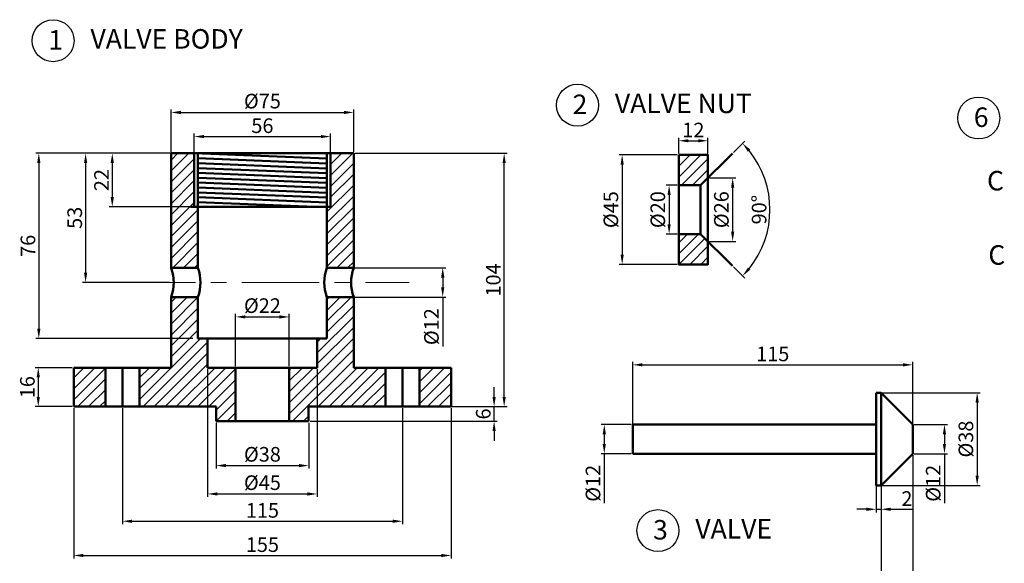
# Model space of a CAD drawing. Units: millimetres. Extents: x 4194 to 4882, y 3816 to 4286.
# Tile 2 of 3: x 4220 to 4624, y 4062 to 4286. Entities that reach past the tile are written whole.
import ezdxf

# ---------------------------------------------------------------- set-up
doc = ezdxf.new("R2010")
doc.units = ezdxf.units.MM
doc.linetypes.add('CENTER', pattern=[50.8, 31.75, -6.35, 6.35, -6.35])
for name, color, linetype, lineweight in [('M-CNTR', 1, 'CENTER', 18), ('M-DIMS', 2, 'Continuous', 25), ('M-HATC', 8, 'Continuous', 18), ('M-OUTL', 7, 'Continuous', 50), ('M-TEXT', 3, 'Continuous', 25)]:
    doc.layers.add(name, color=color, linetype=linetype, lineweight=lineweight)
doc.styles.get("Standard").update_dxf_attribs({"font": 'arial.ttf'})
doc.dimstyles.new('ISO-25', dxfattribs={"dimtxt": 6, "dimasz": 4, "dimexe": 1.25, "dimexo": 0.625, "dimtad": 1, "dimdec": 0, "dimtxsty": 'Standard', "dimcen": 2.5, "dimadec": 0, "dimazin": 0, "dimtfac": 1, "dimtdec": 0, "dimtmove": 0, "dimatfit": 3, "dimfxl": 1, "dimarcsym": 0})

# ---------------------------------------------------------------- blocks, each defined once
blk = doc.blocks.new('*D1')
at = {"layer": 'Defpoints', "color": 0, "transparency": 16777216}
for p in [(4356.86, 4247.5), (4281.86, 4230.74), (4356.86, 4230.74)]:
    blk.add_point(p, dxfattribs=at)
at = {"layer": 'M-DIMS', "color": 0, "lineweight": -2, "transparency": 16777216}
for p, q in [((4281.86, 4231.36), (4281.86, 4248.75)), ((4285.86, 4247.5), (4352.86, 4247.5)), ((4356.86, 4231.36), (4356.86, 4248.75))]:
    blk.add_line(p, q, dxfattribs=at)
at = {"layer": 'M-DIMS', "color": 0, "transparency": 16777216}
for points in [[(4285.86, 4248.17), (4285.86, 4246.83), (4281.86, 4247.5)], [(4352.86, 4248.17), (4352.86, 4246.83), (4356.86, 4247.5)]]:
    blk.add_solid(points, dxfattribs=at)
at = {"layer": 'M-DIMS', "color": 0, "transparency": 16777216, "insert": (4319.36, 4251.36), "char_height": 6, "attachment_point": 5}
blk.add_mtext('%%C75', dxfattribs=at)
blk = doc.blocks.new('*D2')
at = {"layer": 'Defpoints', "color": 0, "transparency": 16777216}
for p in [(4291.36, 4230.74), (4257.69, 4208.74), (4291.36, 4208.74)]:
    blk.add_point(p, dxfattribs=at)
at = {"layer": 'M-DIMS', "color": 0, "lineweight": -2, "transparency": 16777216}
for p, q in [((4290.73, 4230.74), (4256.44, 4230.74)), ((4257.69, 4226.74), (4257.69, 4212.74)), ((4290.73, 4208.74), (4256.44, 4208.74))]:
    blk.add_line(p, q, dxfattribs=at)
at = {"layer": 'M-DIMS', "color": 0, "transparency": 16777216}
for points in [[(4257.02, 4226.74), (4258.36, 4226.74), (4257.69, 4230.74)], [(4257.02, 4212.74), (4258.36, 4212.74), (4257.69, 4208.74)]]:
    blk.add_solid(points, dxfattribs=at)
at = {"layer": 'M-DIMS', "color": 0, "transparency": 16777216, "insert": (4254.05, 4219.74), "char_height": 6, "attachment_point": 5, "rotation": 90}
blk.add_mtext('22', dxfattribs=at)
blk = doc.blocks.new('*D3')
at = {"layer": 'Defpoints', "color": 0, "transparency": 16777216}
for p in [(4281.86, 4230.74), (4227.52, 4154.74), (4291.36, 4154.74)]:
    blk.add_point(p, dxfattribs=at)
at = {"layer": 'M-DIMS', "color": 0, "lineweight": -2, "transparency": 16777216}
for p, q in [((4281.23, 4230.74), (4226.27, 4230.74)), ((4227.52, 4226.74), (4227.52, 4158.74)), ((4290.73, 4154.74), (4226.27, 4154.74))]:
    blk.add_line(p, q, dxfattribs=at)
at = {"layer": 'M-DIMS', "color": 0, "transparency": 16777216}
for points in [[(4226.85, 4226.74), (4228.18, 4226.74), (4227.52, 4230.74)], [(4226.85, 4158.74), (4228.18, 4158.74), (4227.52, 4154.74)]]:
    blk.add_solid(points, dxfattribs=at)
at = {"layer": 'M-DIMS', "color": 0, "transparency": 16777216, "insert": (4223.83, 4192.74), "char_height": 6, "attachment_point": 5, "rotation": 90}
blk.add_mtext('76', dxfattribs=at)
blk = doc.blocks.new('*D8')
at = {"layer": 'Defpoints', "color": 0, "transparency": 16777216}
for p in [(4300.36, 4120.74), (4338.36, 4120.74), (4338.36, 4102.54)]:
    blk.add_point(p, dxfattribs=at)
at = {"layer": 'M-DIMS', "color": 0, "lineweight": -2, "transparency": 16777216}
for p, q in [((4300.36, 4120.11), (4300.36, 4101.29)), ((4338.36, 4120.11), (4338.36, 4101.29)), ((4304.36, 4102.54), (4334.36, 4102.54))]:
    blk.add_line(p, q, dxfattribs=at)
at = {"layer": 'M-DIMS', "color": 0, "transparency": 16777216}
for points in [[(4304.36, 4103.21), (4304.36, 4101.88), (4300.36, 4102.54)], [(4334.36, 4103.21), (4334.36, 4101.88), (4338.36, 4102.54)]]:
    blk.add_solid(points, dxfattribs=at)
at = {"layer": 'M-DIMS', "color": 0, "transparency": 16777216, "insert": (4319.36, 4106.4), "char_height": 6, "attachment_point": 5}
blk.add_mtext('%%C38', dxfattribs=at)
blk = doc.blocks.new('*D9')
at = {"layer": 'Defpoints', "color": 0, "transparency": 16777216}
for p in [(4296.86, 4142.74), (4341.86, 4142.74), (4341.86, 4090.91)]:
    blk.add_point(p, dxfattribs=at)
at = {"layer": 'M-DIMS', "color": 0, "lineweight": -2, "transparency": 16777216}
for p, q in [((4296.86, 4142.11), (4296.86, 4089.66)), ((4341.86, 4142.11), (4341.86, 4089.66)), ((4300.86, 4090.91), (4337.86, 4090.91))]:
    blk.add_line(p, q, dxfattribs=at)
at = {"layer": 'M-DIMS', "color": 0, "transparency": 16777216}
for points in [[(4300.86, 4091.57), (4300.86, 4090.24), (4296.86, 4090.91)], [(4337.86, 4091.57), (4337.86, 4090.24), (4341.86, 4090.91)]]:
    blk.add_solid(points, dxfattribs=at)
at = {"layer": 'M-DIMS', "color": 0, "transparency": 16777216, "insert": (4319.36, 4094.76), "char_height": 6, "attachment_point": 5}
blk.add_mtext('%%C45', dxfattribs=at)
blk = doc.blocks.new('*D10')
at = {"layer": 'Defpoints', "color": 0, "transparency": 16777216}
for p in [(4241.86, 4126.74), (4396.86, 4126.74), (4396.86, 4065.64)]:
    blk.add_point(p, dxfattribs=at)
at = {"layer": 'M-DIMS', "color": 0, "lineweight": -2, "transparency": 16777216}
for p, q in [((4241.86, 4126.11), (4241.86, 4064.39)), ((4396.86, 4126.11), (4396.86, 4064.39)), ((4245.86, 4065.64), (4392.86, 4065.64))]:
    blk.add_line(p, q, dxfattribs=at)
at = {"layer": 'M-DIMS', "color": 0, "transparency": 16777216}
for points in [[(4245.86, 4066.31), (4245.86, 4064.98), (4241.86, 4065.64)], [(4392.86, 4066.31), (4392.86, 4064.98), (4396.86, 4065.64)]]:
    blk.add_solid(points, dxfattribs=at)
at = {"layer": 'M-DIMS', "color": 0, "transparency": 16777216, "insert": (4319.36, 4069.33), "char_height": 6, "attachment_point": 5}
blk.add_mtext('155', dxfattribs=at)
blk = doc.blocks.new('*D11')
at = {"layer": 'Defpoints', "color": 0, "transparency": 16777216}
for p in [(4261.86, 4126.74), (4376.86, 4126.74), (4376.86, 4079.7)]:
    blk.add_point(p, dxfattribs=at)
at = {"layer": 'M-DIMS', "color": 0, "lineweight": -2, "transparency": 16777216}
for p, q in [((4261.86, 4126.11), (4261.86, 4078.45)), ((4376.86, 4126.11), (4376.86, 4078.45)), ((4265.86, 4079.7), (4372.86, 4079.7))]:
    blk.add_line(p, q, dxfattribs=at)
at = {"layer": 'M-DIMS', "color": 0, "transparency": 16777216}
for points in [[(4265.86, 4080.37), (4265.86, 4079.03), (4261.86, 4079.7)], [(4372.86, 4080.37), (4372.86, 4079.03), (4376.86, 4079.7)]]:
    blk.add_solid(points, dxfattribs=at)
at = {"layer": 'M-DIMS', "color": 0, "transparency": 16777216, "insert": (4319.36, 4083.39), "char_height": 6, "attachment_point": 5}
blk.add_mtext('115', dxfattribs=at)
blk = doc.blocks.new('*D12')
at = {"layer": 'Defpoints', "color": 0, "transparency": 16777216}
for p in [(4241.86, 4142.74), (4227.29, 4126.74), (4241.86, 4126.74)]:
    blk.add_point(p, dxfattribs=at)
at = {"layer": 'M-DIMS', "color": 0, "lineweight": -2, "transparency": 16777216}
for p, q in [((4241.23, 4142.74), (4226.04, 4142.74)), ((4227.29, 4138.74), (4227.29, 4130.74)), ((4241.23, 4126.74), (4226.04, 4126.74))]:
    blk.add_line(p, q, dxfattribs=at)
at = {"layer": 'M-DIMS', "color": 0, "transparency": 16777216}
for points in [[(4226.63, 4138.74), (4227.96, 4138.74), (4227.29, 4142.74)], [(4226.63, 4130.74), (4227.96, 4130.74), (4227.29, 4126.74)]]:
    blk.add_solid(points, dxfattribs=at)
at = {"layer": 'M-DIMS', "color": 0, "transparency": 16777216, "insert": (4223.6, 4134.74), "char_height": 6, "attachment_point": 5, "rotation": 90}
blk.add_mtext('16', dxfattribs=at)
blk = doc.blocks.new('*D13')
at = {"layer": 'Defpoints', "color": 0, "transparency": 16777216}
for p in [(4338.36, 4126.74), (4414.53, 4126.74), (4338.36, 4120.74)]:
    blk.add_point(p, dxfattribs=at)
at = {"layer": 'M-DIMS', "color": 0, "lineweight": -2, "transparency": 16777216}
for p, q in [((4414.53, 4130.74), (4414.53, 4134.74)), ((4338.98, 4126.74), (4415.78, 4126.74)), ((4414.53, 4120.74), (4414.53, 4126.74)), ((4338.98, 4120.74), (4415.78, 4120.74)), ((4414.53, 4116.74), (4414.53, 4112.74))]:
    blk.add_line(p, q, dxfattribs=at)
at = {"layer": 'M-DIMS', "color": 0, "transparency": 16777216}
for points in [[(4413.86, 4130.74), (4415.19, 4130.74), (4414.53, 4126.74)], [(4413.86, 4116.74), (4415.19, 4116.74), (4414.53, 4120.74)]]:
    blk.add_solid(points, dxfattribs=at)
at = {"layer": 'M-DIMS', "color": 0, "transparency": 16777216, "insert": (4410.84, 4123.74), "char_height": 6, "attachment_point": 5, "rotation": 90}
blk.add_mtext('6', dxfattribs=at)
blk = doc.blocks.new('*D14')
at = {"layer": 'Defpoints', "color": 0, "transparency": 16777216}
for p in [(4330.36, 4163.58), (4308.36, 4142.74), (4330.36, 4142.74)]:
    blk.add_point(p, dxfattribs=at)
at = {"layer": 'M-DIMS', "color": 0, "lineweight": -2, "transparency": 16777216}
for p, q in [((4308.36, 4143.36), (4308.36, 4164.83)), ((4312.36, 4163.58), (4326.36, 4163.58)), ((4330.36, 4143.36), (4330.36, 4164.83))]:
    blk.add_line(p, q, dxfattribs=at)
at = {"layer": 'M-DIMS', "color": 0, "transparency": 16777216}
for points in [[(4312.36, 4164.24), (4312.36, 4162.91), (4308.36, 4163.58)], [(4326.36, 4164.24), (4326.36, 4162.91), (4330.36, 4163.58)]]:
    blk.add_solid(points, dxfattribs=at)
at = {"layer": 'M-DIMS', "color": 0, "transparency": 16777216, "insert": (4319.36, 4167.43), "char_height": 6, "attachment_point": 5}
blk.add_mtext('%%C22', dxfattribs=at)
blk = doc.blocks.new('*D15')
at = {"layer": 'Defpoints', "color": 0, "transparency": 16777216}
for p in [(4356.86, 4230.74), (4418.66, 4230.74), (4405.21, 4126.74)]:
    blk.add_point(p, dxfattribs=at)
at = {"layer": 'M-DIMS', "color": 0, "lineweight": -2, "transparency": 16777216}
for p, q in [((4357.48, 4230.74), (4419.91, 4230.74)), ((4418.66, 4130.74), (4418.66, 4226.74)), ((4405.84, 4126.74), (4419.91, 4126.74))]:
    blk.add_line(p, q, dxfattribs=at)
at = {"layer": 'M-DIMS', "color": 0, "transparency": 16777216}
for points in [[(4417.99, 4226.74), (4419.33, 4226.74), (4418.66, 4230.74)], [(4417.99, 4130.74), (4419.33, 4130.74), (4418.66, 4126.74)]]:
    blk.add_solid(points, dxfattribs=at)
at = {"layer": 'M-DIMS', "color": 0, "transparency": 16777216, "insert": (4414.97, 4178.74), "char_height": 6, "attachment_point": 5, "rotation": 90}
blk.add_mtext('104', dxfattribs=at)
blk = doc.blocks.new('*D16')
at = {"layer": 'Defpoints', "color": 0, "transparency": 16777216}
for p in [(4281.86, 4230.74), (4246.74, 4177.74), (4281.86, 4177.74)]:
    blk.add_point(p, dxfattribs=at)
at = {"layer": 'M-DIMS', "color": 0, "lineweight": -2, "transparency": 16777216}
for p, q in [((4281.23, 4230.74), (4245.49, 4230.74)), ((4246.74, 4226.74), (4246.74, 4181.74)), ((4281.23, 4177.74), (4245.49, 4177.74))]:
    blk.add_line(p, q, dxfattribs=at)
at = {"layer": 'M-DIMS', "color": 0, "transparency": 16777216}
for points in [[(4246.07, 4226.74), (4247.4, 4226.74), (4246.74, 4230.74)], [(4246.07, 4181.74), (4247.4, 4181.74), (4246.74, 4177.74)]]:
    blk.add_solid(points, dxfattribs=at)
at = {"layer": 'M-DIMS', "color": 0, "transparency": 16777216, "insert": (4243.04, 4204.24), "char_height": 6, "attachment_point": 5, "rotation": 90}
blk.add_mtext('53', dxfattribs=at)
blk = doc.blocks.new('*D17')
at = {"layer": 'Defpoints', "color": 0, "transparency": 16777216}
for p in [(4356.86, 4183.74), (4356.86, 4171.74), (4393.42, 4171.74)]:
    blk.add_point(p, dxfattribs=at)
at = {"layer": 'M-DIMS', "color": 0, "lineweight": -2, "transparency": 16777216}
for p, q in [((4357.48, 4183.74), (4394.67, 4183.74)), ((4393.42, 4179.74), (4393.42, 4175.74)), ((4357.48, 4171.74), (4394.67, 4171.74)), ((4393.42, 4171.74), (4393.42, 4151.43))]:
    blk.add_line(p, q, dxfattribs=at)
at = {"layer": 'M-DIMS', "color": 0, "transparency": 16777216}
for points in [[(4392.75, 4179.74), (4394.09, 4179.74), (4393.42, 4183.74)], [(4392.75, 4175.74), (4394.09, 4175.74), (4393.42, 4171.74)]]:
    blk.add_solid(points, dxfattribs=at)
at = {"layer": 'M-DIMS', "color": 0, "transparency": 16777216, "insert": (4389.56, 4159.58), "char_height": 6, "attachment_point": 5, "rotation": 90}
blk.add_mtext('%%C12', dxfattribs=at)
blk = doc.blocks.new('*D18')
at = {"layer": 'Defpoints', "color": 0, "transparency": 16777216}
for p in [(4347.36, 4237.59), (4291.36, 4230.74), (4347.36, 4230.74)]:
    blk.add_point(p, dxfattribs=at)
at = {"layer": 'M-DIMS', "color": 0, "lineweight": -2, "transparency": 16777216}
for p, q in [((4291.36, 4231.36), (4291.36, 4238.84)), ((4347.36, 4231.36), (4347.36, 4238.84)), ((4295.36, 4237.59), (4343.36, 4237.59))]:
    blk.add_line(p, q, dxfattribs=at)
at = {"layer": 'M-DIMS', "color": 0, "transparency": 16777216}
for points in [[(4295.36, 4238.26), (4295.36, 4236.93), (4291.36, 4237.59)], [(4343.36, 4238.26), (4343.36, 4236.93), (4347.36, 4237.59)]]:
    blk.add_solid(points, dxfattribs=at)
at = {"layer": 'M-DIMS', "color": 0, "transparency": 16777216, "insert": (4319.36, 4241.28), "char_height": 6, "attachment_point": 5}
blk.add_mtext('56', dxfattribs=at)
blk = doc.blocks.new('*D20')
at = {"layer": 'Defpoints', "color": 0, "transparency": 16777216}
for p in [(4502.37, 4220.59), (4502.37, 4194.59), (4512.5, 4194.59)]:
    blk.add_point(p, dxfattribs=at)
at = {"layer": 'M-DIMS', "color": 0, "lineweight": -2, "transparency": 16777216}
for p, q in [((4502.99, 4220.59), (4513.75, 4220.59)), ((4512.5, 4216.59), (4512.5, 4198.59)), ((4502.99, 4194.59), (4513.75, 4194.59))]:
    blk.add_line(p, q, dxfattribs=at)
at = {"layer": 'M-DIMS', "color": 0, "transparency": 16777216}
for points in [[(4511.84, 4216.59), (4513.17, 4216.59), (4512.5, 4220.59)], [(4511.84, 4198.59), (4513.17, 4198.59), (4512.5, 4194.59)]]:
    blk.add_solid(points, dxfattribs=at)
at = {"layer": 'M-DIMS', "color": 0, "transparency": 16777216, "insert": (4508.65, 4207.59), "char_height": 6, "attachment_point": 5, "rotation": 90}
blk.add_mtext('%%C26', dxfattribs=at)
blk = doc.blocks.new('*D21')
at = {"layer": 'Defpoints', "color": 0, "transparency": 16777216}
for p in [(4512.41, 4230.64), (4499.37, 4217.59), (4499.37, 4197.59), (4526.53, 4197.63), (4512.41, 4184.54)]:
    blk.add_point(p, dxfattribs=at)
at = {"layer": 'M-DIMS', "color": 0, "lineweight": -2, "transparency": 16777216}
for p, q in [((4512.85, 4231.08), (4517.45, 4235.68)), ((4512.85, 4184.1), (4517.45, 4179.5))]:
    blk.add_line(p, q, dxfattribs=at)
blk.add_arc((4489.37, 4207.59), 38.47, 320.9601, 39.0399, dxfattribs=at)
at = {"layer": 'M-DIMS', "color": 0, "transparency": 16777216}
for points in [[(4518.75, 4231.37), (4519.74, 4232.27), (4516.57, 4234.79)], [(4519.74, 4182.91), (4518.75, 4183.8), (4516.57, 4180.39)]]:
    blk.add_solid(points, dxfattribs=at)
at = {"layer": 'M-DIMS', "color": 0, "transparency": 16777216, "insert": (4524.15, 4207.59), "char_height": 6, "attachment_point": 5, "rotation": 90}
blk.add_mtext('90°', dxfattribs=at)
blk = doc.blocks.new('*D22')
at = {"layer": 'Defpoints', "color": 0, "transparency": 16777216}
for p in [(4502.37, 4235.88), (4490.37, 4230.09), (4502.37, 4230.09)]:
    blk.add_point(p, dxfattribs=at)
at = {"layer": 'M-DIMS', "color": 0, "lineweight": -2, "transparency": 16777216}
for p, q in [((4490.37, 4230.71), (4490.37, 4237.13)), ((4494.37, 4235.88), (4498.37, 4235.88)), ((4502.37, 4230.71), (4502.37, 4237.13))]:
    blk.add_line(p, q, dxfattribs=at)
at = {"layer": 'M-DIMS', "color": 0, "transparency": 16777216}
for points in [[(4494.37, 4236.54), (4494.37, 4235.21), (4490.37, 4235.88)], [(4498.37, 4236.54), (4498.37, 4235.21), (4502.37, 4235.88)]]:
    blk.add_solid(points, dxfattribs=at)
at = {"layer": 'M-DIMS', "color": 0, "transparency": 16777216, "insert": (4496.37, 4239.51), "char_height": 6, "attachment_point": 5}
blk.add_mtext('12', dxfattribs=at)
blk = doc.blocks.new('*D23')
at = {"layer": 'Defpoints', "color": 0, "transparency": 16777216}
for p in [(4490.37, 4217.59), (4486.41, 4197.59), (4490.37, 4197.59)]:
    blk.add_point(p, dxfattribs=at)
at = {"layer": 'M-DIMS', "color": 0, "lineweight": -2, "transparency": 16777216}
for p, q in [((4489.74, 4217.59), (4485.16, 4217.59)), ((4486.41, 4213.59), (4486.41, 4201.59)), ((4489.74, 4197.59), (4485.16, 4197.59))]:
    blk.add_line(p, q, dxfattribs=at)
at = {"layer": 'M-DIMS', "color": 0, "transparency": 16777216}
for points in [[(4485.74, 4213.59), (4487.08, 4213.59), (4486.41, 4217.59)], [(4485.74, 4201.59), (4487.08, 4201.59), (4486.41, 4197.59)]]:
    blk.add_solid(points, dxfattribs=at)
at = {"layer": 'M-DIMS', "color": 0, "transparency": 16777216, "insert": (4482.55, 4207.59), "char_height": 6, "attachment_point": 5, "rotation": 90}
blk.add_mtext('%%C20', dxfattribs=at)
blk = doc.blocks.new('*D24')
at = {"layer": 'Defpoints', "color": 0, "transparency": 16777216}
for p in [(4490.37, 4230.09), (4467.12, 4185.12), (4490.37, 4185.12)]:
    blk.add_point(p, dxfattribs=at)
at = {"layer": 'M-DIMS', "color": 0, "lineweight": -2, "transparency": 16777216}
for p, q in [((4489.74, 4230.09), (4465.87, 4230.09)), ((4467.12, 4226.09), (4467.12, 4189.12)), ((4489.74, 4185.12), (4465.87, 4185.12))]:
    blk.add_line(p, q, dxfattribs=at)
at = {"layer": 'M-DIMS', "color": 0, "transparency": 16777216}
for points in [[(4466.46, 4226.09), (4467.79, 4226.09), (4467.12, 4230.09)], [(4466.46, 4189.12), (4467.79, 4189.12), (4467.12, 4185.12)]]:
    blk.add_solid(points, dxfattribs=at)
at = {"layer": 'M-DIMS', "color": 0, "transparency": 16777216, "insert": (4463.27, 4207.6), "char_height": 6, "attachment_point": 5, "rotation": 90}
blk.add_mtext('%%C45', dxfattribs=at)
blk = doc.blocks.new('*D25')
at = {"layer": 'Defpoints', "color": 0, "transparency": 16777216}
for p in [(4471.46, 4119.44), (4459.79, 4107.44), (4471.46, 4107.44)]:
    blk.add_point(p, dxfattribs=at)
at = {"layer": 'M-DIMS', "color": 0, "lineweight": -2, "transparency": 16777216}
for p, q in [((4470.84, 4119.44), (4458.54, 4119.44)), ((4459.79, 4115.44), (4459.79, 4111.44)), ((4470.84, 4107.44), (4458.54, 4107.44)), ((4459.79, 4107.44), (4459.79, 4087.13))]:
    blk.add_line(p, q, dxfattribs=at)
at = {"layer": 'M-DIMS', "color": 0, "transparency": 16777216}
for points in [[(4459.12, 4115.44), (4460.45, 4115.44), (4459.79, 4119.44)], [(4459.12, 4111.44), (4460.45, 4111.44), (4459.79, 4107.44)]]:
    blk.add_solid(points, dxfattribs=at)
at = {"layer": 'M-DIMS', "color": 0, "transparency": 16777216, "insert": (4455.93, 4095.28), "char_height": 6, "attachment_point": 5, "rotation": 90}
blk.add_mtext('%%C12', dxfattribs=at)
blk = doc.blocks.new('*D26')
at = {"layer": 'Defpoints', "color": 0, "transparency": 16777216}
for p in [(4586.46, 4143.91), (4471.46, 4115.35), (4586.46, 4113.44)]:
    blk.add_point(p, dxfattribs=at)
at = {"layer": 'M-DIMS', "color": 0, "lineweight": -2, "transparency": 16777216}
for p, q in [((4471.46, 4115.97), (4471.46, 4145.16)), ((4475.46, 4143.91), (4582.46, 4143.91)), ((4586.46, 4114.06), (4586.46, 4145.16))]:
    blk.add_line(p, q, dxfattribs=at)
at = {"layer": 'M-DIMS', "color": 0, "transparency": 16777216}
for points in [[(4475.46, 4144.58), (4475.46, 4143.25), (4471.46, 4143.91)], [(4582.46, 4144.58), (4582.46, 4143.25), (4586.46, 4143.91)]]:
    blk.add_solid(points, dxfattribs=at)
at = {"layer": 'M-DIMS', "color": 0, "transparency": 16777216, "insert": (4528.96, 4147.6), "char_height": 6, "attachment_point": 5}
blk.add_mtext('115', dxfattribs=at)
blk = doc.blocks.new('*D27')
at = {"layer": 'Defpoints', "color": 0, "transparency": 16777216}
for p in [(4573.46, 4113.44), (4571.46, 4112.1), (4573.46, 4084.61)]:
    blk.add_point(p, dxfattribs=at)
at = {"layer": 'M-DIMS', "color": 0, "lineweight": -2, "transparency": 16777216}
for p, q in [((4571.46, 4111.47), (4571.46, 4083.36)), ((4573.46, 4112.81), (4573.46, 4083.36)), ((4567.46, 4084.61), (4563.46, 4084.61)), ((4571.46, 4084.61), (4573.46, 4084.61)), ((4577.46, 4084.61), (4586.69, 4084.61))]:
    blk.add_line(p, q, dxfattribs=at)
at = {"layer": 'M-DIMS', "color": 0, "transparency": 16777216}
for points in [[(4567.46, 4085.28), (4567.46, 4083.94), (4571.46, 4084.61)], [(4577.46, 4085.28), (4577.46, 4083.94), (4573.46, 4084.61)]]:
    blk.add_solid(points, dxfattribs=at)
at = {"layer": 'M-DIMS', "color": 0, "transparency": 16777216, "insert": (4584.07, 4088.25), "char_height": 6, "attachment_point": 5}
blk.add_mtext('2', dxfattribs=at)
blk = doc.blocks.new('*D28')
at = {"layer": 'Defpoints', "color": 0, "transparency": 16777216}
for p in [(4586.46, 4119.44), (4586.46, 4107.44), (4599.51, 4107.44)]:
    blk.add_point(p, dxfattribs=at)
at = {"layer": 'M-DIMS', "color": 0, "lineweight": -2, "transparency": 16777216}
for p, q in [((4587.09, 4119.44), (4600.76, 4119.44)), ((4599.51, 4115.44), (4599.51, 4111.44)), ((4587.09, 4107.44), (4600.76, 4107.44)), ((4599.51, 4107.44), (4599.51, 4087.13))]:
    blk.add_line(p, q, dxfattribs=at)
at = {"layer": 'M-DIMS', "color": 0, "transparency": 16777216}
for points in [[(4598.84, 4115.44), (4600.17, 4115.44), (4599.51, 4119.44)], [(4598.84, 4111.44), (4600.17, 4111.44), (4599.51, 4107.44)]]:
    blk.add_solid(points, dxfattribs=at)
at = {"layer": 'M-DIMS', "color": 0, "transparency": 16777216, "insert": (4595.65, 4095.28), "char_height": 6, "attachment_point": 5, "rotation": 90}
blk.add_mtext('%%C12', dxfattribs=at)
blk = doc.blocks.new('*D29')
at = {"layer": 'Defpoints', "color": 0, "transparency": 16777216}
for p in [(4573.46, 4132.44), (4572.46, 4094.44), (4612.94, 4094.44)]:
    blk.add_point(p, dxfattribs=at)
at = {"layer": 'M-DIMS', "color": 0, "lineweight": -2, "transparency": 16777216}
for p, q in [((4574.09, 4132.44), (4614.19, 4132.44)), ((4612.94, 4128.44), (4612.94, 4098.44)), ((4573.09, 4094.44), (4614.19, 4094.44))]:
    blk.add_line(p, q, dxfattribs=at)
at = {"layer": 'M-DIMS', "color": 0, "transparency": 16777216}
for points in [[(4612.27, 4128.44), (4613.6, 4128.44), (4612.94, 4132.44)], [(4612.27, 4098.44), (4613.6, 4098.44), (4612.94, 4094.44)]]:
    blk.add_solid(points, dxfattribs=at)
at = {"layer": 'M-DIMS', "color": 0, "transparency": 16777216, "insert": (4609.08, 4113.44), "char_height": 6, "attachment_point": 5, "rotation": 90}
blk.add_mtext('%%C38', dxfattribs=at)
blk = doc.blocks.new('*D52')
at = {"layer": 'Defpoints', "color": 0, "transparency": 16777216}
for p in [(4586.46, 4107.44), (4573.46, 4094.44), (4586.46, 3817.63)]:
    blk.add_point(p, dxfattribs=at)
at = {"layer": 'M-DIMS', "color": 0, "lineweight": -2, "transparency": 16777216}
for p, q in [((4586.46, 4106.81), (4586.46, 3816.38)), ((4573.46, 4093.81), (4573.46, 3816.38)), ((4577.46, 3817.63), (4582.46, 3817.63))]:
    blk.add_line(p, q, dxfattribs=at)
at = {"layer": 'M-DIMS', "color": 0, "transparency": 16777216}
for points in [[(4577.46, 3818.3), (4577.46, 3816.97), (4573.46, 3817.63)], [(4582.46, 3818.3), (4582.46, 3816.97), (4586.46, 3817.63)]]:
    blk.add_solid(points, dxfattribs=at)
at = {"layer": 'M-DIMS', "color": 0, "transparency": 16777216, "insert": (4579.96, 3821.32), "char_height": 6, "attachment_point": 5}
blk.add_mtext('13', dxfattribs=at)

msp = doc.modelspace()

# ---------------------------------------------------------------- hatches: boundary and pattern name
at = {"layer": 'M-HATC'}
h = msp.add_hatch(dxfattribs=at)
h.set_pattern_fill('ANSI31', color=256)
h.paths.add_polyline_path([(4502.366, 4185.0895), (4502.366, 4194.5895), (4499.366, 4197.5895), (4490.366, 4197.5895), (4490.366, 4185.0895)], flags=17)
h.paths.add_polyline_path([(4291.358, 4230.7397), (4281.858, 4230.7397), (4281.858, 4183.7397), (4292.858, 4183.7397), (4292.858, 4208.7397), (4291.358, 4208.7397)])
h.paths.add_polyline_path([(4356.858, 4230.7397), (4347.358, 4230.7397), (4347.358, 4208.7397), (4345.858, 4208.7397), (4345.858, 4183.7397), (4356.858, 4183.7397)])
h.paths.add_polyline_path([(4356.858, 4142.7397), (4356.858, 4171.7397), (4345.858, 4171.7397), (4345.858, 4154.7397), (4341.858, 4154.7397), (4341.858, 4142.7397), (4330.358, 4142.7397), (4330.358, 4120.7397), (4338.358, 4120.7397), (4338.358, 4126.7397), (4369.858, 4126.7397), (4369.858, 4142.7397)])
h.paths.add_polyline_path([(4300.358, 4126.7397), (4300.358, 4120.7397), (4308.358, 4120.7397), (4308.358, 4142.7397), (4296.858, 4142.7397), (4296.858, 4154.7397), (4292.858, 4154.7397), (4292.858, 4171.7397), (4281.858, 4171.7397), (4281.858, 4142.7397), (4268.858, 4142.7397), (4268.858, 4126.7397)])
h.paths.add_polyline_path([(4254.858, 4126.7397), (4254.858, 4142.7397), (4241.858, 4142.7397), (4241.858, 4126.7397)])
h.paths.add_polyline_path([(4396.858, 4126.7397), (4396.858, 4142.7397), (4383.858, 4142.7397), (4383.858, 4126.7397)])
h.paths.add_polyline_path([(4502.366, 4194.5895), (4499.366, 4197.5895), (4490.366, 4197.5895), (4490.366, 4185.0895), (4502.366, 4185.0895)])
h = msp.add_hatch(dxfattribs=at)
h.set_pattern_fill('ANSI31', color=256)
h.paths.add_polyline_path([(4502.366, 4230.0895), (4490.366, 4230.0895), (4490.366, 4217.5895), (4499.366, 4217.5895), (4502.366, 4220.5895)])
h.paths.add_polyline_path([(4502.366, 4194.5895), (4499.366, 4197.5895), (4490.366, 4197.5895), (4490.366, 4185.0895), (4502.366, 4185.0895)])

# ---------------------------------------------------------------- linework, layer by layer
at = {"layer": 'M-CNTR'}
msp.add_line((4260.1033, 4177.7397), (4379.5832, 4177.7397), dxfattribs=at)
at = {"layer": 'M-OUTL'}
for p, q in [((4281.858, 4230.7397), (4356.858, 4230.7397)), ((4281.858, 4183.7397), (4281.858, 4230.7397)), ((4291.358, 4230.7397), (4345.858, 4228.5459)), ((4291.358, 4208.7397), (4291.358, 4230.7397)), ((4292.858, 4183.7397), (4292.858, 4230.7397)), ((4345.858, 4183.7397), (4345.858, 4230.7397)), ((4347.358, 4208.7397), (4347.358, 4230.7397)), ((4356.858, 4183.7397), (4356.858, 4230.7397)), ((4499.366, 4217.5895), (4512.4124, 4230.6359)), ((4292.858, 4228.6793), (4345.858, 4226.5459)), ((4292.858, 4226.6793), (4345.858, 4224.5459)), ((4292.858, 4224.6793), (4345.858, 4222.5459)), ((4292.858, 4222.6793), (4345.858, 4220.5459)), ((4292.858, 4220.6793), (4345.858, 4218.5459)), ((4292.858, 4218.6793), (4345.858, 4216.5459)), ((4292.858, 4216.6793), (4345.858, 4214.5459)), ((4292.858, 4214.6793), (4345.858, 4212.5459)), ((4490.366, 4217.5895), (4499.366, 4217.5895)), ((4499.366, 4197.5895), (4499.366, 4217.5895)), ((4292.858, 4212.6793), (4345.858, 4210.5459)), ((4292.858, 4210.6793), (4341.0445, 4208.7397)), ((4289.858, 4208.7397), (4347.358, 4208.7397)), ((4490.366, 4197.5895), (4499.366, 4197.5895)), ((4499.366, 4197.5895), (4512.4124, 4184.5431)), ((4281.858, 4183.7397), (4292.858, 4183.7397)), ((4345.858, 4183.7397), (4356.858, 4183.7397)), ((4281.858, 4142.7397), (4281.858, 4171.7397)), ((4281.858, 4171.7397), (4292.858, 4171.7397)), ((4292.858, 4154.7397), (4292.858, 4171.7397)), ((4345.858, 4171.7397), (4356.858, 4171.7397)), ((4345.858, 4154.7397), (4345.858, 4171.7397)), ((4356.858, 4142.7397), (4356.858, 4171.7397)), ((4292.858, 4154.7397), (4345.858, 4154.7397)), ((4296.858, 4142.7397), (4296.858, 4154.7397)), ((4341.858, 4142.7397), (4341.858, 4154.7397)), ((4281.858, 4142.7397), (4241.858, 4142.7397)), ((4241.858, 4126.7397), (4241.858, 4142.7397)), ((4254.858, 4126.7397), (4254.858, 4142.7397)), ((4261.858, 4126.7397), (4261.858, 4142.7397)), ((4268.858, 4126.7397), (4268.858, 4142.7397)), ((4296.858, 4142.7397), (4341.858, 4142.7397)), ((4308.358, 4120.7397), (4308.358, 4142.7397)), ((4330.358, 4120.7397), (4330.358, 4142.7397)), ((4396.858, 4142.7397), (4356.858, 4142.7397)), ((4369.858, 4126.7397), (4369.858, 4142.7397)), ((4376.858, 4126.7397), (4376.858, 4142.7397)), ((4383.858, 4126.7397), (4383.858, 4142.7397)), ((4396.858, 4126.7397), (4396.858, 4142.7397)), ((4571.4627, 4094.4374), (4571.4627, 4132.4374)), ((4571.4627, 4132.4374), (4573.4627, 4132.4374)), ((4573.4627, 4094.4374), (4573.4627, 4132.4374)), ((4586.4627, 4119.4374), (4573.4627, 4132.4374)), ((4241.858, 4126.7397), (4300.358, 4126.7397)), ((4300.358, 4120.7397), (4300.358, 4126.7397)), ((4338.358, 4126.7397), (4396.858, 4126.7397)), ((4338.358, 4120.7397), (4338.358, 4126.7397)), ((4300.358, 4120.7397), (4338.358, 4120.7397)), ((4471.4627, 4119.4374), (4571.4627, 4119.4374)), ((4471.4627, 4107.4374), (4471.4627, 4119.4374)), ((4586.4627, 4107.4374), (4586.4627, 4119.4374)), ((4471.4627, 4107.4374), (4571.4627, 4107.4374)), ((4573.4627, 4094.4374), (4586.4627, 4107.4374)), ((4571.4627, 4094.4374), (4573.4627, 4094.4374))]:
    msp.add_line(p, q, dxfattribs=at)
msp.add_lwpolyline([(4490.366, 4230.0895), (4502.366, 4230.0895), (4502.366, 4185.0895), (4490.366, 4185.0895)], close=True, dxfattribs=at)
for centre, start, end in [((4265.4656, 4177.7397), 339.896091, 20.103909), ((4276.4656, 4177.7397), 339.896091, 20.103909), ((4362.2503, 4177.7397), 159.896091, 200.103909), ((4373.2503, 4177.7397), 159.896091, 200.103909)]:
    msp.add_arc(centre, 17.4559, start, end, dxfattribs=at)
at = {"layer": 'M-TEXT'}
for centre in [(4233.385, 4276.9439), (4448.7686, 4250.4736), (4613.5632, 4245.2154), (4481.8232, 4075.8681)]:
    msp.add_circle(centre, 8.6164, dxfattribs=at)

# ---------------------------------------------------------------- texts
at = {"layer": 'M-TEXT', "char_height": 8}
for s, width, insert, attachment_point in [('1', 8, (4231.3829, 4281.2821), 1), ('VALVE BODY', 117.140838, (4248.7365, 4281.6921), 1), ('2', 8, (4446.7665, 4254.8118), 1), ('VALVE NUT', 64.226233, (4464.1201, 4255.2218), 1), ('6', 8, (4611.5611, 4249.5537), 1), ('C', 8, (4616.9721, 4223.4904), 1), ('C', 8, (4624.4772, 4192.9948), 3), ('VALVE', 38.884897, (4497.1747, 4080.6163), 1), ('3', 8, (4479.8211, 4080.2064), 1)]:
    msp.add_mtext_dynamic_manual_height_columns(s, width=width, gutter_width=12.5, heights=[0], dxfattribs=dict(at, insert=insert, attachment_point=attachment_point))

# ---------------------------------------------------------------- dimensions: what is measured, and where the dimension line sits
at = {"layer": 'M-DIMS'}
for base, p1, p2, text, picture, middle in [((4356.858, 4247.499), (4281.858, 4230.7397), (4356.858, 4230.7397), '%%C<>', '*D1', (4319.358, 4251.3552)), ((4330.358, 4163.5763), (4308.358, 4142.7397), (4330.358, 4142.7397), '%%C<>', '*D14', (4319.358, 4167.4325)), ((4341.858, 4090.9053), (4296.858, 4142.7397), (4341.858, 4142.7397), '%%C45', '*D9', (4319.358, 4094.7615)), ((4338.358, 4102.5441), (4300.358, 4120.7397), (4338.358, 4120.7397), '%%C<>', '*D8', (4319.358, 4106.4004))]:
    dim = msp.add_linear_dim(base=base, p1=p1, p2=p2, text=text, dimstyle='ISO-25', override={"dimclrd": 0, "dimclre": 0, "dimclrt": 0}, dxfattribs=at)
    dim.commit()
    dim.dimension.update_dxf_attribs({"geometry": picture, "text_midpoint": middle})
for base, p1, p2, override, picture, middle in [((4347.358, 4237.594), (4291.358, 4230.7397), (4347.358, 4230.7397), {"dimclrd": 0, "dimclre": 0, "dimclrt": 0}, '*D18', (4319.358, 4241.2824)), ((4502.366, 4235.8763), (4490.366, 4230.0895), (4502.366, 4230.0895), {"dimclrd": 0, "dimclre": 0, "dimclrt": 0}, '*D22', (4496.366, 4239.5136)), ((4586.4627, 4143.9145), (4471.4627, 4115.3452), (4586.4627, 4113.4374), {"dimclrd": 0, "dimclre": 0, "dimclrt": 0}, '*D26', (4528.9627, 4147.603)), ((4396.858, 4065.6423), (4241.858, 4126.7397), (4396.858, 4126.7397), {"dimclrd": 0, "dimclre": 0, "dimclrt": 0}, '*D10', (4319.358, 4069.3307)), ((4376.858, 4079.7011), (4261.858, 4126.7397), (4376.858, 4126.7397), {"dimclrd": 0, "dimclre": 0, "dimclrt": 0}, '*D11', (4319.358, 4083.3896)), ((4573.4627, 4084.6115), (4571.4627, 4112.0987), (4573.4627, 4113.4374), {"dimclrd": 0, "dimclre": 0, "dimclrt": 0}, '*D27', (4584.0748, 4088.2488)), ((4586.4627, 3817.6331), (4573.4627, 4094.4374), (4586.4627, 4107.4374), {"dimdec": 0, "dimlfac": 1, "dimrnd": 0, "dimzin": 0, "dimdsep": 46, "dimlunit": 2}, '*D52', (4579.9627, 3821.3236))]:
    dim = msp.add_linear_dim(base=base, p1=p1, p2=p2, dimstyle='ISO-25', override=override, dxfattribs=at)
    dim.commit()
    dim.dimension.update_dxf_attribs({"geometry": picture, "text_midpoint": middle})
dim = msp.add_angular_dim_2l(base=(4526.5253, 4197.6327), line1=((4499.366, 4197.5895), (4512.4124, 4184.5431)), line2=((4499.366, 4217.5895), (4512.4124, 4230.6359)), dimstyle='ISO-25', override={"dimclrd": 0, "dimclre": 0, "dimclrt": 0}, dxfattribs=at)
dim.commit()
dim.dimension.update_dxf_attribs({"geometry": '*D21', "text_midpoint": (4524.1477, 4207.5895)})
for base, p1, p2, picture, middle in [((4227.5178, 4154.7397), (4281.858, 4230.7397), (4291.358, 4154.7397), '*D3', (4223.8294, 4192.7397)), ((4246.7355, 4177.7397), (4281.858, 4230.7397), (4281.858, 4177.7397), '*D16', (4243.045, 4204.2397)), ((4257.6908, 4208.7397), (4291.358, 4230.7397), (4291.358, 4208.7397), '*D2', (4254.0535, 4219.7397)), ((4418.6598, 4230.7397), (4405.2123, 4126.7397), (4356.858, 4230.7397), '*D15', (4414.9713, 4178.7397)), ((4227.2932, 4126.7397), (4241.858, 4142.7397), (4241.858, 4126.7397), '*D12', (4223.6047, 4134.7397)), ((4414.5275, 4126.7397), (4338.358, 4120.7397), (4338.358, 4126.7397), '*D13', (4410.8391, 4123.7397))]:
    dim = msp.add_linear_dim(base=base, p1=p1, p2=p2, angle=90, dimstyle='ISO-25', override={"dimclrd": 0, "dimclre": 0, "dimclrt": 0}, dxfattribs=at)
    dim.commit()
    dim.dimension.update_dxf_attribs({"geometry": picture, "text_midpoint": middle})
for base, p1, p2, picture, middle in [((4467.1242, 4185.1201), (4490.366, 4230.0895), (4490.366, 4185.1201), '*D24', (4463.268, 4207.6048)), ((4512.5037, 4194.5895), (4502.366, 4220.5895), (4502.366, 4194.5895), '*D20', (4508.6475, 4207.5895)), ((4486.4105, 4197.5895), (4490.366, 4217.5895), (4490.366, 4197.5895), '*D23', (4482.5543, 4207.5895)), ((4393.4197, 4171.7397), (4356.858, 4183.7397), (4356.858, 4171.7397), '*D17', (4389.5635, 4159.584)), ((4612.9373, 4094.4374), (4573.4627, 4132.4374), (4572.4627, 4094.4374), '*D29', (4609.081, 4113.4374)), ((4459.7866, 4107.4374), (4471.4627, 4119.4374), (4471.4627, 4107.4374), '*D25', (4455.9303, 4095.2817)), ((4599.5068, 4107.4374), (4586.4627, 4119.4374), (4586.4627, 4107.4374), '*D28', (4595.6506, 4095.2817))]:
    dim = msp.add_linear_dim(base=base, p1=p1, p2=p2, angle=90, text='%%C<>', dimstyle='ISO-25', override={"dimclrd": 0, "dimclre": 0, "dimclrt": 0}, dxfattribs=at)
    dim.commit()
    dim.dimension.update_dxf_attribs({"geometry": picture, "text_midpoint": middle})

doc.saveas('drawing.dxf')
